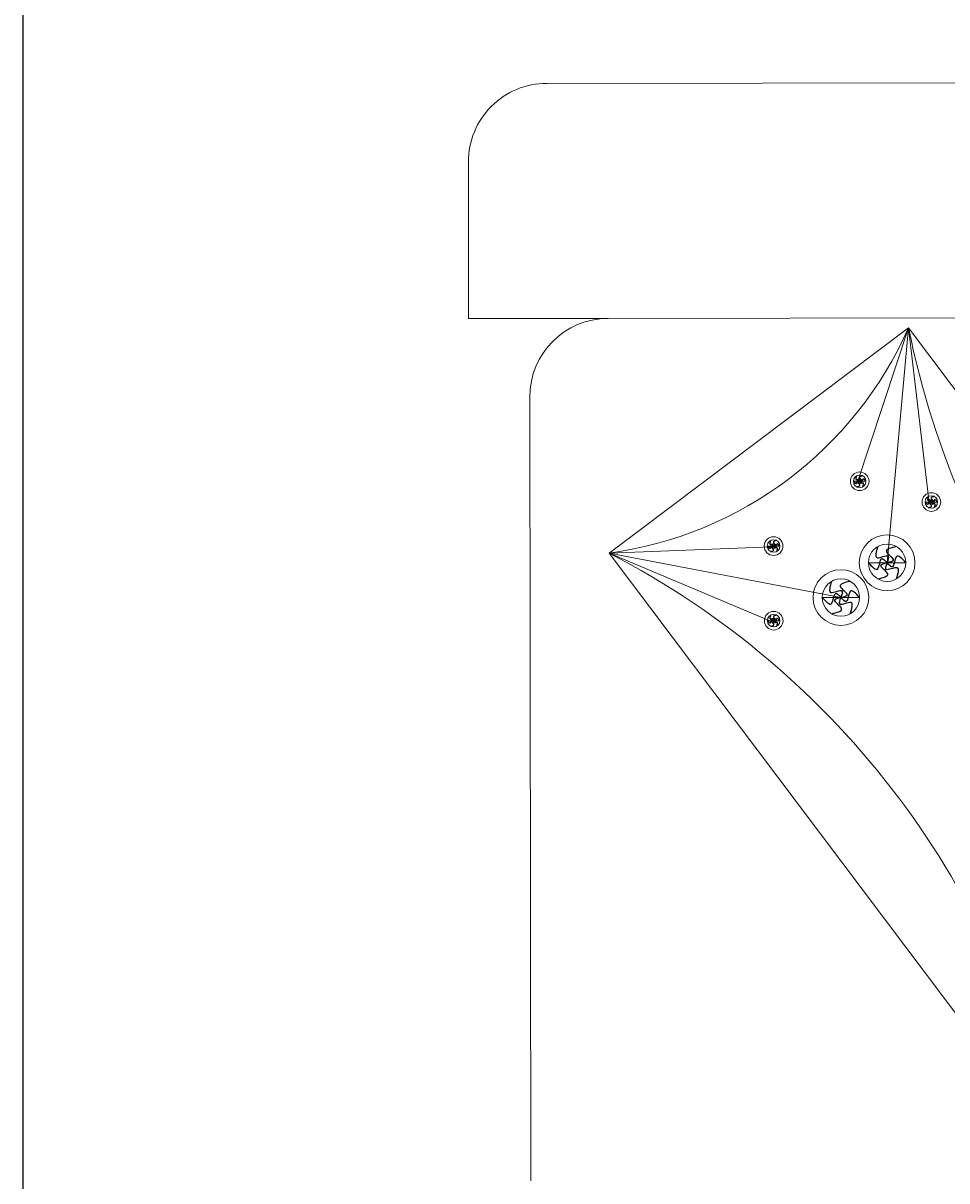
# Model space of a CAD drawing. Units: inches. Extents: x -61 to 1599, y -1316 to 257.
# Tile 138 of 204: x 492 to 515, y -104 to -74. Entities that reach past the tile are written whole.
import ezdxf

# ---------------------------------------------------------------- set-up
doc = ezdxf.new("R2010")
doc.units = ezdxf.units.IN
doc.header["$MEASUREMENT"] = 0
doc.layers.add('A-ANNO-DIMS', color=2, linetype='Continuous', lineweight=18)
doc.layers.add('FURNITURE', color=83, linetype='Continuous', lineweight=18)
doc.layers.add('FUR', color=83, linetype='Continuous')
doc.styles.get("Standard").update_dxf_attribs({"font": 'arial.ttf'})
doc.dimstyles.get("Standard").update_dxf_attribs({"dimtxt": 0.18, "dimasz": 0.18, "dimexe": 0.18, "dimexo": 0.0625, "dimgap": 0.09, "dimtad": 0, "dimtih": 1, "dimtoh": 1, "dimdec": 0, "dimzin": 0, "dimdsep": 46, "dimlunit": 3, "dimtxsty": 'Standard', "dimcen": 0.09, "dimadec": 0, "dimazin": 0, "dimtfac": 1, "dimtdec": 0, "dimtofl": 0, "dimtmove": 0, "dimatfit": 3, "dimfxl": 1, "dimtolj": 1, "dimtzin": 0, "dimarcsym": 0})

# ---------------------------------------------------------------- blocks, each defined once
blk = doc.blocks.new('*U246')
at = {"layer": 'FUR'}
blk.add_open_spline([(0.005, 0.08), (-0.03, 0.048), (-0.098, -0.015), (0.075, -0.018), (0.024, -0.063), (0.005, -0.08)], degree=3, knots=[0, 0, 0, 0, 0.0954578, 0.1898773, 0.2470677, 0.2470677, 0.2470677, 0.2470677], dxfattribs=at)
blk = doc.blocks.new('*U247')
at = {"layer": 'FURNITURE', "transparency": 16777216}
for p, rotation in [((222.173, -79.977), 60), ((222.178, -80.056), 120), ((222.25, -80.092), 180), ((222.312, -79.968), 300), ((222.317, -80.048), 240)]:
    blk.add_blockref('*U246', p, dxfattribs=dict(at, rotation=rotation))
blk.add_blockref('*U246', (222.24, -79.932), dxfattribs=at)
blk = doc.blocks.new('*U248')
at = {"layer": 'FUR'}
blk.add_open_spline([(0.005, 0.08), (-0.03, 0.048), (-0.098, -0.015), (0.075, -0.018), (0.024, -0.063), (0.005, -0.08)], degree=3, knots=[0, 0, 0, 0, 0.0954578, 0.1898773, 0.2470677, 0.2470677, 0.2470677, 0.2470677], dxfattribs=at)
blk = doc.blocks.new('*U249')
at = {"layer": 'FURNITURE', "transparency": 16777216}
for p, rotation in [((222.173, -79.977), 60), ((222.178, -80.056), 120), ((222.25, -80.092), 180), ((222.312, -79.968), 300), ((222.317, -80.048), 240)]:
    blk.add_blockref('*U248', p, dxfattribs=dict(at, rotation=rotation))
blk.add_blockref('*U248', (222.24, -79.932), dxfattribs=at)
blk = doc.blocks.new('*U250')
at = {"layer": 'FUR'}
blk.add_open_spline([(0.005, 0.08), (-0.03, 0.048), (-0.098, -0.015), (0.075, -0.018), (0.024, -0.063), (0.005, -0.08)], degree=3, knots=[0, 0, 0, 0, 0.0954578, 0.1898773, 0.2470677, 0.2470677, 0.2470677, 0.2470677], dxfattribs=at)
blk = doc.blocks.new('*U238')
at = {"layer": 'FURNITURE', "transparency": 16777216}
for p, rotation in [((222.173, -79.977), 60), ((222.178, -80.056), 120), ((222.25, -80.092), 180), ((222.312, -79.968), 300), ((222.317, -80.048), 240)]:
    blk.add_blockref('*U250', p, dxfattribs=dict(at, rotation=rotation))
blk.add_blockref('*U250', (222.24, -79.932), dxfattribs=at)
blk = doc.blocks.new('*U239')
at = {"layer": 'FUR'}
blk.add_open_spline([(0.005, 0.08), (-0.03, 0.048), (-0.098, -0.015), (0.075, -0.018), (0.024, -0.063), (0.005, -0.08)], degree=3, knots=[0, 0, 0, 0, 0.0954578, 0.1898773, 0.2470677, 0.2470677, 0.2470677, 0.2470677], dxfattribs=at)
blk = doc.blocks.new('*U240')
at = {"layer": 'FURNITURE', "transparency": 16777216}
for p, rotation in [((222.173, -79.977), 60), ((222.178, -80.056), 120), ((222.25, -80.092), 180), ((222.312, -79.968), 300), ((222.317, -80.048), 240)]:
    blk.add_blockref('*U239', p, dxfattribs=dict(at, rotation=rotation))
blk.add_blockref('*U239', (222.24, -79.932), dxfattribs=at)
blk = doc.blocks.new('*U211')
at = {"layer": 'FUR'}
blk.add_open_spline([(0.015, 0.238), (-0.088, 0.143), (-0.292, -0.045), (0.224, -0.053), (0.072, -0.187), (0.015, -0.238)], degree=3, knots=[0, 0, 0, 0, 0.2846533, 0.5662105, 0.736751, 0.736751, 0.736751, 0.736751], dxfattribs=at)
blk = doc.blocks.new('*U212')
at = {"layer": 'FURNITURE', "transparency": 16777216}
for p, rotation in [((662.517, -238.489), 60), ((662.929, -238.463), 300), ((662.531, -238.727), 120), ((662.745, -238.833), 180), ((662.944, -238.702), 240)]:
    blk.add_blockref('*U211', p, dxfattribs=dict(at, rotation=rotation))
blk.add_blockref('*U211', (662.716, -238.357), dxfattribs=at)
blk = doc.blocks.new('*U251')
at = {"layer": 'FUR'}
blk.add_open_spline([(0.015, 0.238), (-0.088, 0.143), (-0.292, -0.045), (0.224, -0.053), (0.072, -0.187), (0.015, -0.238)], degree=3, knots=[0, 0, 0, 0, 0.2846533, 0.5662105, 0.736751, 0.736751, 0.736751, 0.736751], dxfattribs=at)
blk = doc.blocks.new('*U237')
at = {"layer": 'FURNITURE', "transparency": 16777216}
for p, rotation in [((662.517, -238.489), 60), ((662.929, -238.463), 300), ((662.531, -238.727), 120), ((662.745, -238.833), 180), ((662.944, -238.702), 240)]:
    blk.add_blockref('*U251', p, dxfattribs=dict(at, rotation=rotation))
blk.add_blockref('*U251', (662.716, -238.357), dxfattribs=at)
blk = doc.blocks.new('*D704')
at = {"layer": 'A-ANNO-DIMS', "color": 0, "lineweight": -2, "transparency": 16777216}
for p, q in [((491.833, -616.882), (491.833, 257.457)), ((492.013, 257.277), (517.874, 257.277)), ((544.523, 257.277), (518.661, 257.277)), ((544.703, -616.882), (544.703, 257.457))]:
    blk.add_line(p, q, dxfattribs=at)
at = {"layer": 'A-ANNO-DIMS', "color": 0, "transparency": 16777216}
for points in [[(492.013, 257.307), (492.013, 257.247), (491.833, 257.277)], [(544.523, 257.307), (544.523, 257.247), (544.703, 257.277)]]:
    blk.add_solid(points, dxfattribs=at)
at = {"layer": 'DEFPOINTS', "color": 0, "transparency": 16777216}
for p in [(544.703, 257.277), (491.833, -616.945), (544.703, -616.945)]:
    blk.add_point(p, dxfattribs=at)
at = {"layer": 'A-ANNO-DIMS', "color": 0, "transparency": 16777216, "insert": (518.268, 257.277), "char_height": 0.18, "attachment_point": 5}
blk.add_mtext('\\A1;52.87', dxfattribs=at)

msp = doc.modelspace()

# ---------------------------------------------------------------- linework, layer by layer
at = {"layer": 'FURNITURE'}
for p, q in [((506.7579, -81.8149), (503.1999, -81.8197)), ((506.7579, -81.8149), (523.7299, -81.7915)), ((514.4247, -82.0531), (513.1247, -85.9885)), ((514.4247, -82.0531), (513.8773, -88.0479)), ((514.4247, -82.0531), (514.9538, -86.5181)), ((504.7607, -83.8176), (504.7882, -103.8176)), ((513.1772, -85.9691), (513.0174, -85.9693)), ((513.1772, -85.9691), (513.337, -85.9689)), ((515.0062, -86.4987), (514.8464, -86.4989)), ((515.0062, -86.4987), (515.166, -86.4984)), ((506.7866, -87.8015), (510.9281, -87.6417)), ((510.9805, -87.6223), (510.8207, -87.6225)), ((510.9805, -87.6223), (511.1403, -87.6221)), ((506.7866, -87.8015), (512.6987, -88.9349)), ((506.7866, -87.8015), (510.9307, -89.5458)), ((513.8773, -88.0479), (513.4008, -88.0485)), ((513.8773, -88.0479), (514.3538, -88.0472)), ((512.6987, -88.9349), (512.2222, -88.9356)), ((512.6987, -88.9349), (513.1752, -88.9342)), ((510.9831, -89.5264), (510.8233, -89.5266)), ((510.9831, -89.5264), (511.1429, -89.5262))]:
    msp.add_line(p, q, dxfattribs=at)
msp.add_lwpolyline([(503.2659, -129.8197), (503.2714, -133.8197, 0.4142136), (505.2742, -135.817), (527.2741, -135.7867, 0.4142137), (529.2714, -133.784), (529.1944, -77.784, 0.4142134), (527.1916, -75.7868), (505.1917, -75.817, 0.4142136), (503.1944, -77.8197), (503.1999, -81.8197)], format="xyb", dxfattribs=at)
msp.add_lwpolyline([(518.1128, -102.851), (506.7866, -87.8015), (514.4247, -82.0531), (525.7509, -97.1025)], close=True, dxfattribs=at)
for centre, radius in [((513.1772, -85.9691), 0.2382), ((513.1772, -85.9691), 0.1598), ((515.0062, -86.4987), 0.2382), ((515.0062, -86.4987), 0.1598), ((510.9805, -87.6223), 0.2382), ((513.8773, -88.0479), 0.7104), ((510.9805, -87.6223), 0.1598), ((513.8773, -88.0479), 0.4765), ((512.6987, -88.9349), 0.7104), ((512.6987, -88.9349), 0.4765), ((510.9831, -89.5264), 0.2382), ((510.9831, -89.5264), 0.1598)]:
    msp.add_circle(centre, radius, dxfattribs=at)
for centre, radius, start, end in [((506.7607, -83.8148), 2, 90.07876, 180.07876), ((505.45, -78.0769), 9.816, 277.82577, 336.10452), ((535.7357, -77.8012), 21.731, 191.28318, 242.64711), ((496.8019, -107.1028), 21.731, 11.28318, 62.64711)]:
    msp.add_arc(centre, radius, start, end, dxfattribs=at)

# ---------------------------------------------------------------- block references
at = {"layer": 'FURNITURE', "rotation": 270.0787336990067}
for name, p in [('*U238', (592.884, 136.3856)), ('*U240', (594.713, 135.856)), ('*U247', (590.6874, 134.7324)), ('*U237', (751.5615, 575.0095)), ('*U212', (750.383, 574.1225)), ('*U249', (590.69, 132.8283))]:
    msp.add_blockref(name, p, dxfattribs=at)

# ---------------------------------------------------------------- dimensions: what is measured, and where the dimension line sits
at = {"layer": 'A-ANNO-DIMS'}
dim = msp.add_linear_dim(base=(544.7028, 257.2771), p1=(491.8327, -616.9446), p2=(544.7028, -616.9446), dimstyle='Standard', override={"dimdec": 2, "dimlfac": 1, "dimrnd": 0, "dimzin": 0, "dimdsep": 46, "dimlunit": 2}, dxfattribs=at)
dim.commit()
dim.dimension.update_dxf_attribs({"geometry": '*D704', "text_midpoint": (518.2677, 257.2771)})

doc.saveas('drawing.dxf')
